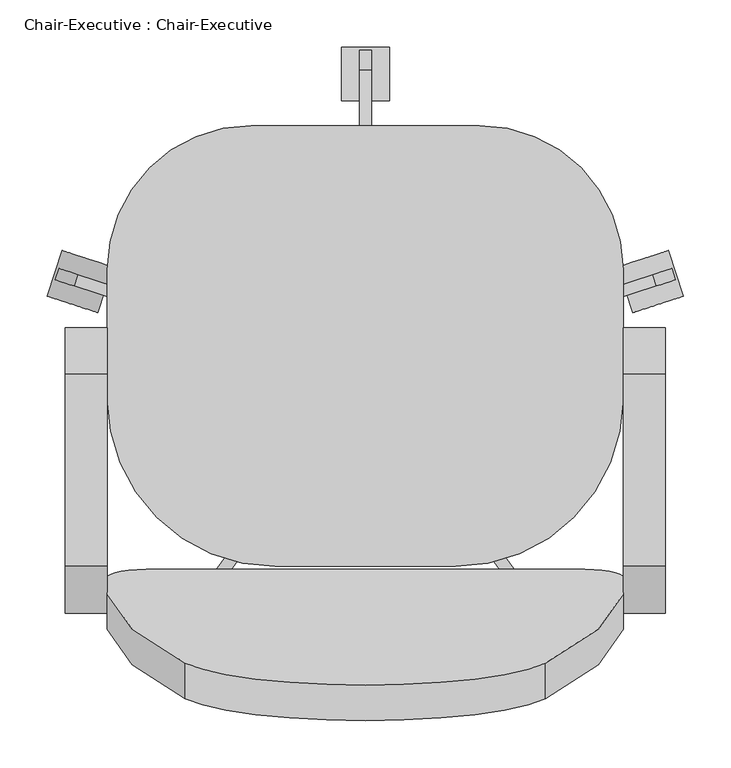
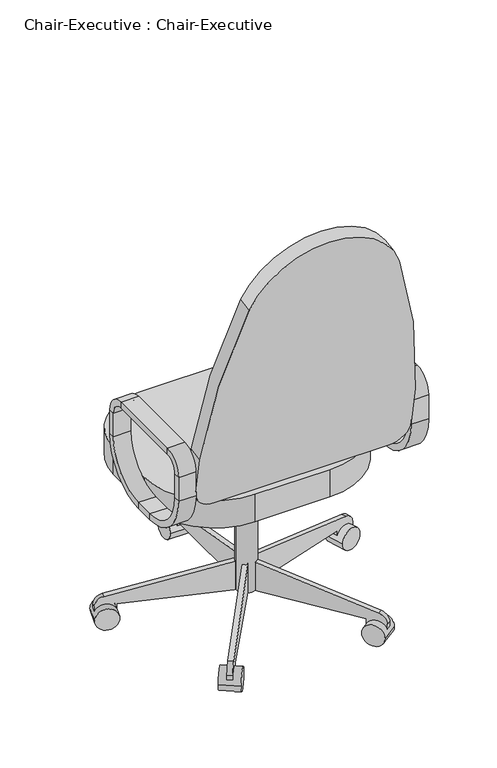
"""IFC4 building model written with IfcOpenShell, lengths in millimetres: furniture geometry, Chair-Executive : Chair-Executive."""

from ifc_helpers import new_model, si_unit, point, frame, frame_2d, origin, place, context, project, spatial, polyline, circle_curve, trimmed, segment, composite_curve, outline, extrude, source, transform, mapped, element, save
from ifc_brep_helpers import plane_surface, cylinder_surface, revolved_surface, advanced_brep


def chair_executive_chair_executive_8d69e98c(model_context):
    return source(origin(), model_context, "Body", "SolidModel", [
        advanced_brep(
        [(-176.5091803, -217.7873012, 546.1), (-176.5091803, -108.0540984, 436.3667972), (-176.5091803, -108.0540984, 420.4917972), (-176.5091803, -233.6623012, 546.1), (-132.0591803, -217.7873012, 546.1), (-132.0591803, -108.0540984, 436.3667972), (-132.0591803, -233.6623012, 546.1), (-132.0591803, -108.0540984, 420.4917972), (-176.5091803, -233.6623012, 609.6), (-176.5091803, -217.7873012, 609.6), (-132.0591803, -217.7873012, 609.6), (-132.0591803, -233.6623012, 609.6), (-176.5091803, -184.2540984, 643.1332028), (-176.5091803, -184.2540984, 659.0082028), (-132.0591803, -184.2540984, 643.1332028), (-132.0591803, -184.2540984, 659.0082028), (-176.5091803, 18.9459016, 659.0082028), (-176.5091803, 18.9459016, 643.1332028), (-132.0591803, 18.9459016, 643.1332028), (-132.0591803, 18.9459016, 659.0082028), (-176.5091803, 52.4791044, 609.6), (-176.5091803, 68.3541044, 609.6), (-132.0591803, 52.4791044, 609.6), (-132.0591803, 68.3541044, 609.6), (-176.5091803, 68.3541044, 546.1), (-176.5091803, 52.4791044, 546.1), (-132.0591803, 52.4791044, 546.1), (-132.0591803, 68.3541044, 546.1), (-176.5091803, -57.2540984, 436.3667972), (-176.5091803, -57.2540984, 420.4917972), (-132.0591803, -57.2540984, 436.3667972), (-132.0591803, -57.2540984, 420.4917972)],
        [
            (0, 1, circle_curve(frame((-176.5091803, -108.0540984, 546.1), z_axis=(1.0, 0.0, 0.0), x_axis=(0.0, 0.0, -1.0)), 109.7332028)),
            (1, 2),
            (2, 3, circle_curve(frame((-176.5091803, -108.0540984, 546.1), z_axis=(-1.0, 0.0, 0.0), x_axis=(0.0, 0.0, -1.0)), 125.6082028)),
            (3, 0),
            (4, 5, circle_curve(frame((-132.0591803, -108.0540984, 546.1), z_axis=(1.0, 0.0, 0.0), x_axis=(0.0, 0.0, -1.0)), 109.7332028)),
            (5, 1),
            (0, 4),
            (6, 7, circle_curve(frame((-132.0591803, -108.0540984, 546.1), z_axis=(1.0, 0.0, 0.0), x_axis=(0.0, 0.0, -1.0)), 125.6082028)),
            (7, 5),
            (4, 6),
            (2, 7),
            (6, 3),
            (3, 8),
            (8, 9),
            (9, 0),
            (9, 10),
            (10, 4),
            (10, 11),
            (11, 6),
            (11, 8),
            (12, 9, circle_curve(frame((-176.5091803, -184.2540984, 609.6), z_axis=(1.0, 0.0, 0.0), x_axis=(0.0, -1.0, 0.0)), 33.5332028)),
            (8, 13, circle_curve(frame((-176.5091803, -184.2540984, 609.6), z_axis=(-1.0, 0.0, 0.0), x_axis=(0.0, -1.0, 0.0)), 49.4082028)),
            (13, 12),
            (14, 10, circle_curve(frame((-132.0591803, -184.2540984, 609.6), z_axis=(1.0, 0.0, 0.0), x_axis=(0.0, -1.0, 0.0)), 33.5332028)),
            (12, 14),
            (15, 11, circle_curve(frame((-132.0591803, -184.2540984, 609.6), z_axis=(1.0, 0.0, 0.0), x_axis=(0.0, -1.0, 0.0)), 49.4082028)),
            (14, 15),
            (15, 13),
            (13, 16),
            (16, 17),
            (17, 12),
            (17, 18),
            (18, 14),
            (18, 19),
            (19, 15),
            (19, 16),
            (20, 17, circle_curve(frame((-176.5091803, 18.9459016, 609.6), z_axis=(1.0, 0.0, 0.0), x_axis=(0.0, 0.0, 1.0)), 33.5332028)),
            (16, 21, circle_curve(frame((-176.5091803, 18.9459016, 609.6), z_axis=(-1.0, 0.0, 0.0), x_axis=(0.0, 0.0, 1.0)), 49.4082028)),
            (21, 20),
            (22, 18, circle_curve(frame((-132.0591803, 18.9459016, 609.6), z_axis=(1.0, 0.0, 0.0), x_axis=(0.0, 0.0, 1.0)), 33.5332028)),
            (20, 22),
            (23, 19, circle_curve(frame((-132.0591803, 18.9459016, 609.6), z_axis=(1.0, 0.0, 0.0), x_axis=(0.0, 0.0, 1.0)), 49.4082028)),
            (22, 23),
            (23, 21),
            (21, 24),
            (24, 25),
            (25, 20),
            (25, 26),
            (26, 22),
            (26, 27),
            (27, 23),
            (27, 24),
            (28, 25, circle_curve(frame((-176.5091803, -57.2540984, 546.1), z_axis=(1.0, 0.0, 0.0), x_axis=(0.0, 1.0, 0.0)), 109.7332028)),
            (24, 29, circle_curve(frame((-176.5091803, -57.2540984, 546.1), z_axis=(-1.0, 0.0, 0.0), x_axis=(0.0, 1.0, 0.0)), 125.6082028)),
            (29, 28),
            (30, 26, circle_curve(frame((-132.0591803, -57.2540984, 546.1), z_axis=(1.0, 0.0, 0.0), x_axis=(0.0, 1.0, 0.0)), 109.7332028)),
            (28, 30),
            (31, 27, circle_curve(frame((-132.0591803, -57.2540984, 546.1), z_axis=(1.0, 0.0, 0.0), x_axis=(0.0, 1.0, 0.0)), 125.6082028)),
            (30, 31),
            (31, 29),
            (29, 2),
            (1, 28),
            (5, 30),
            (7, 31),
        ],
        [
            plane_surface(frame((-176.5091803, -108.0540984, 546.1), z_axis=(-1.0, 0.0, 0.0), x_axis=(0.0, 0.0, -1.0))),
            revolved_surface(polyline([(-176.5091803, -108.0540984, 436.3667972), (-132.0591803, -108.0540984, 436.3667972)]), (-132.0591803, -108.0540984, 546.1), (-1.0, 0.0, 0.0)),
            plane_surface(frame((-132.0591803, -108.0540984, 546.1), z_axis=(1.0, 0.0, 0.0), x_axis=(0.0, 0.0, -1.0))),
            cylinder_surface(frame((-132.0591803, -108.0540984, 546.1), z_axis=(-1.0, 0.0, 0.0), x_axis=(0.0, 0.0, -1.0)), 125.6082028),
            plane_surface(frame((-176.5091803, -233.6623012, 546.1), z_axis=(-1.0, 0.0, 0.0), x_axis=(0.0, 0.0, 1.0))),
            plane_surface(frame((-176.5091803, -217.7873012, 546.1), z_axis=(0.0, 1.0, 0.0), x_axis=(0.0, 0.0, 1.0))),
            plane_surface(frame((-132.0591803, -217.7873012, 546.1), z_axis=(1.0, 0.0, 0.0), x_axis=(0.0, 0.0, 1.0))),
            plane_surface(frame((-132.0591803, -233.6623012, 546.1), z_axis=(0.0, -1.0, 0.0), x_axis=(0.0, 0.0, 1.0))),
            plane_surface(frame((-176.5091803, -184.2540984, 609.6), z_axis=(-1.0, 0.0, 0.0), x_axis=(0.0, -1.0, 0.0))),
            revolved_surface(polyline([(-176.5091803, -217.7873012, 609.6), (-132.0591803, -217.7873012, 609.6)]), (-132.0591803, -184.2540984, 609.6), (-1.0, 0.0, 0.0)),
            plane_surface(frame((-132.0591803, -184.2540984, 609.6), z_axis=(1.0, 0.0, 0.0), x_axis=(0.0, -1.0, 0.0))),
            cylinder_surface(frame((-132.0591803, -184.2540984, 609.6), z_axis=(-1.0, 0.0, 0.0), x_axis=(0.0, -1.0, 0.0)), 49.4082028),
            plane_surface(frame((-176.5091803, -184.2540984, 659.0082028), z_axis=(-1.0, 0.0, 0.0), x_axis=(0.0, 1.0, 0.0))),
            plane_surface(frame((-176.5091803, -184.2540984, 643.1332028), z_axis=(0.0, 0.0, -1.0), x_axis=(0.0, 1.0, 0.0))),
            plane_surface(frame((-132.0591803, -184.2540984, 643.1332028), z_axis=(1.0, 0.0, 0.0), x_axis=(0.0, 1.0, 0.0))),
            plane_surface(frame((-132.0591803, -184.2540984, 659.0082028), z_axis=(0.0, 0.0, 1.0), x_axis=(0.0, 1.0, 0.0))),
            plane_surface(frame((-176.5091803, 18.9459016, 609.6), z_axis=(-1.0, 0.0, 0.0), x_axis=(0.0, 0.0, 1.0))),
            revolved_surface(polyline([(-176.5091803, 18.9459016, 643.1332028), (-132.0591803, 18.9459016, 643.1332028)]), (-132.0591803, 18.9459016, 609.6), (-1.0, 0.0, 0.0)),
            plane_surface(frame((-132.0591803, 18.9459016, 609.6), z_axis=(1.0, 0.0, 0.0), x_axis=(0.0, 0.0, 1.0))),
            cylinder_surface(frame((-132.0591803, 18.9459016, 609.6), z_axis=(-1.0, 0.0, 0.0), x_axis=(0.0, 0.0, 1.0)), 49.4082028),
            plane_surface(frame((-176.5091803, 68.3541044, 609.6), z_axis=(-1.0, 0.0, 0.0), x_axis=(0.0, 0.0, -1.0))),
            plane_surface(frame((-176.5091803, 52.4791044, 609.6), z_axis=(0.0, -1.0, 0.0), x_axis=(0.0, 0.0, -1.0))),
            plane_surface(frame((-132.0591803, 52.4791044, 609.6), z_axis=(1.0, 0.0, 0.0), x_axis=(0.0, 0.0, -1.0))),
            plane_surface(frame((-132.0591803, 68.3541044, 609.6), z_axis=(0.0, 1.0, 0.0), x_axis=(0.0, 0.0, -1.0))),
            plane_surface(frame((-176.5091803, -57.2540984, 546.1), z_axis=(-1.0, 0.0, 0.0), x_axis=(0.0, 1.0, 0.0))),
            revolved_surface(polyline([(-176.5091803, 52.479104400000004, 546.1), (-132.0591803, 52.479104400000004, 546.1)]), (-132.0591803, -57.2540984, 546.1), (-1.0, 0.0, 0.0)),
            plane_surface(frame((-132.0591803, -57.2540984, 546.1), z_axis=(1.0, 0.0, 0.0), x_axis=(0.0, 1.0, 0.0))),
            cylinder_surface(frame((-132.0591803, -57.2540984, 546.1), z_axis=(-1.0, 0.0, 0.0), x_axis=(0.0, 1.0, 0.0)), 125.6082028),
            plane_surface(frame((-176.5091803, -57.2540984, 420.4917972), z_axis=(-1.0, 0.0, 0.0), x_axis=(0.0, -1.0, 0.0))),
            plane_surface(frame((-176.5091803, -57.2540984, 436.3667972), z_axis=(0.0, 0.0, 1.0), x_axis=(0.0, -1.0, 0.0))),
            plane_surface(frame((-132.0591803, -57.2540984, 436.3667972), z_axis=(1.0, 0.0, 0.0), x_axis=(0.0, -1.0, 0.0))),
            plane_surface(frame((-132.0591803, -57.2540984, 420.4917972), z_axis=(0.0, 0.0, -1.0), x_axis=(0.0, -1.0, 0.0))),
        ],
        [
            (0, [[1, 2, 3, 4]]),
            (1, [[5, 6, -1, 7]]),
            (2, [[8, 9, -5, 10]]),
            (3, [[-3, 11, -8, 12]]),
            (4, [[-4, 13, 14, 15]]),
            (5, [[-7, -15, 16, 17]]),
            (6, [[-10, -17, 18, 19]]),
            (7, [[-12, -19, 20, -13]]),
            (8, [[21, -14, 22, 23]]),
            (9, [[24, -16, -21, 25]]),
            (10, [[26, -18, -24, 27]]),
            (11, [[-22, -20, -26, 28]]),
            (12, [[-23, 29, 30, 31]]),
            (13, [[-25, -31, 32, 33]]),
            (14, [[-27, -33, 34, 35]]),
            (15, [[-28, -35, 36, -29]]),
            (16, [[37, -30, 38, 39]]),
            (17, [[40, -32, -37, 41]]),
            (18, [[42, -34, -40, 43]]),
            (19, [[-38, -36, -42, 44]]),
            (20, [[-39, 45, 46, 47]]),
            (21, [[-41, -47, 48, 49]]),
            (22, [[-43, -49, 50, 51]]),
            (23, [[-44, -51, 52, -45]]),
            (24, [[53, -46, 54, 55]]),
            (25, [[56, -48, -53, 57]]),
            (26, [[58, -50, -56, 59]]),
            (27, [[-54, -52, -58, 60]]),
            (28, [[-55, 61, -2, 62]]),
            (29, [[-57, -62, -6, 63]]),
            (30, [[-59, -63, -9, 64]]),
            (31, [[-60, -64, -11, -61]]),
        ],
    ),
        advanced_brep(
        [(414.0408197, -233.6623012, 546.1), (414.0408197, -108.0540984, 420.4917972), (458.4908197, -108.0540984, 420.4917972), (458.4908197, -233.6623012, 546.1), (414.0408197, -217.7873012, 546.1), (414.0408197, -108.0540984, 436.3667972), (458.4908197, -217.7873012, 546.1), (458.4908197, -108.0540984, 436.3667972), (458.4908197, -233.6623012, 609.6), (414.0408197, -233.6623012, 609.6), (414.0408197, -217.7873012, 609.6), (458.4908197, -217.7873012, 609.6), (414.0408197, -184.2540984, 659.0082028), (458.4908197, -184.2540984, 659.0082028), (414.0408197, -184.2540984, 643.1332028), (458.4908197, -184.2540984, 643.1332028), (458.4908197, 18.9459016, 659.0082028), (414.0408197, 18.9459016, 659.0082028), (414.0408197, 18.9459016, 643.1332028), (458.4908197, 18.9459016, 643.1332028), (414.0408197, 68.3541044, 609.6), (458.4908197, 68.3541044, 609.6), (414.0408197, 52.4791044, 609.6), (458.4908197, 52.4791044, 609.6), (458.4908197, 68.3541044, 546.1), (414.0408197, 68.3541044, 546.1), (414.0408197, 52.4791044, 546.1), (458.4908197, 52.4791044, 546.1), (414.0408197, -57.2540984, 420.4917972), (458.4908197, -57.2540984, 420.4917972), (414.0408197, -57.2540984, 436.3667972), (458.4908197, -57.2540984, 436.3667972)],
        [
            (0, 1, circle_curve(frame((414.0408197, -108.0540984, 546.1), z_axis=(1.0, 0.0, 0.0), x_axis=(0.0, 0.0, -1.0)), 125.6082028)),
            (1, 2),
            (2, 3, circle_curve(frame((458.4908197, -108.0540984, 546.1), z_axis=(-1.0, 0.0, 0.0), x_axis=(0.0, 0.0, -1.0)), 125.6082028)),
            (3, 0),
            (4, 5, circle_curve(frame((414.0408197, -108.0540984, 546.1), z_axis=(1.0, 0.0, 0.0), x_axis=(0.0, 0.0, -1.0)), 109.7332028)),
            (5, 1),
            (0, 4),
            (6, 7, circle_curve(frame((458.4908197, -108.0540984, 546.1), z_axis=(1.0, 0.0, 0.0), x_axis=(0.0, 0.0, -1.0)), 109.7332028)),
            (7, 5),
            (4, 6),
            (2, 7),
            (6, 3),
            (3, 8),
            (8, 9),
            (9, 0),
            (9, 10),
            (10, 4),
            (10, 11),
            (11, 6),
            (11, 8),
            (12, 9, circle_curve(frame((414.0408197, -184.2540984, 609.6), z_axis=(1.0, 0.0, 0.0), x_axis=(0.0, -1.0, 0.0)), 49.4082028)),
            (8, 13, circle_curve(frame((458.4908197, -184.2540984, 609.6), z_axis=(-1.0, 0.0, 0.0), x_axis=(0.0, -1.0, 0.0)), 49.4082028)),
            (13, 12),
            (14, 10, circle_curve(frame((414.0408197, -184.2540984, 609.6), z_axis=(1.0, 0.0, 0.0), x_axis=(0.0, -1.0, 0.0)), 33.5332028)),
            (12, 14),
            (15, 11, circle_curve(frame((458.4908197, -184.2540984, 609.6), z_axis=(1.0, 0.0, 0.0), x_axis=(0.0, -1.0, 0.0)), 33.5332028)),
            (14, 15),
            (15, 13),
            (13, 16),
            (16, 17),
            (17, 12),
            (17, 18),
            (18, 14),
            (18, 19),
            (19, 15),
            (19, 16),
            (20, 17, circle_curve(frame((414.0408197, 18.9459016, 609.6), z_axis=(1.0, 0.0, 0.0), x_axis=(0.0, 0.0, 1.0)), 49.4082028)),
            (16, 21, circle_curve(frame((458.4908197, 18.9459016, 609.6), z_axis=(-1.0, 0.0, 0.0), x_axis=(0.0, 0.0, 1.0)), 49.4082028)),
            (21, 20),
            (22, 18, circle_curve(frame((414.0408197, 18.9459016, 609.6), z_axis=(1.0, 0.0, 0.0), x_axis=(0.0, 0.0, 1.0)), 33.5332028)),
            (20, 22),
            (23, 19, circle_curve(frame((458.4908197, 18.9459016, 609.6), z_axis=(1.0, 0.0, 0.0), x_axis=(0.0, 0.0, 1.0)), 33.5332028)),
            (22, 23),
            (23, 21),
            (21, 24),
            (24, 25),
            (25, 20),
            (25, 26),
            (26, 22),
            (26, 27),
            (27, 23),
            (27, 24),
            (28, 25, circle_curve(frame((414.0408197, -57.2540984, 546.1), z_axis=(1.0, 0.0, 0.0), x_axis=(0.0, 1.0, 0.0)), 125.6082028)),
            (24, 29, circle_curve(frame((458.4908197, -57.2540984, 546.1), z_axis=(-1.0, 0.0, 0.0), x_axis=(0.0, 1.0, 0.0)), 125.6082028)),
            (29, 28),
            (30, 26, circle_curve(frame((414.0408197, -57.2540984, 546.1), z_axis=(1.0, 0.0, 0.0), x_axis=(0.0, 1.0, 0.0)), 109.7332028)),
            (28, 30),
            (31, 27, circle_curve(frame((458.4908197, -57.2540984, 546.1), z_axis=(1.0, 0.0, 0.0), x_axis=(0.0, 1.0, 0.0)), 109.7332028)),
            (30, 31),
            (31, 29),
            (29, 2),
            (1, 28),
            (5, 30),
            (7, 31),
        ],
        [
            cylinder_surface(frame((414.0408197, -108.0540984, 546.1), z_axis=(-1.0, 0.0, 0.0), x_axis=(0.0, 0.0, -1.0)), 125.6082028),
            plane_surface(frame((414.0408197, -108.0540984, 546.1), z_axis=(-1.0, 0.0, 0.0), x_axis=(0.0, 0.0, -1.0))),
            revolved_surface(polyline([(414.0408197, -108.0540984, 436.3667972), (458.4908197, -108.0540984, 436.3667972)]), (414.0408197, -108.0540984, 546.1), (-1.0, 0.0, 0.0)),
            plane_surface(frame((458.4908197, -108.0540984, 546.1), z_axis=(1.0, 0.0, 0.0), x_axis=(0.0, 0.0, -1.0))),
            plane_surface(frame((458.4908197, -233.6623012, 546.1), z_axis=(0.0, -1.0, 0.0), x_axis=(0.0, 0.0, 1.0))),
            plane_surface(frame((414.0408197, -233.6623012, 546.1), z_axis=(-1.0, 0.0, 0.0), x_axis=(0.0, 0.0, 1.0))),
            plane_surface(frame((414.0408197, -217.7873012, 546.1), z_axis=(0.0, 1.0, 0.0), x_axis=(0.0, 0.0, 1.0))),
            plane_surface(frame((458.4908197, -217.7873012, 546.1), z_axis=(1.0, 0.0, 0.0), x_axis=(0.0, 0.0, 1.0))),
            cylinder_surface(frame((414.0408197, -184.2540984, 609.6), z_axis=(-1.0, 0.0, 0.0), x_axis=(0.0, -1.0, 0.0)), 49.4082028),
            plane_surface(frame((414.0408197, -184.2540984, 609.6), z_axis=(-1.0, 0.0, 0.0), x_axis=(0.0, -1.0, 0.0))),
            revolved_surface(polyline([(414.0408197, -217.7873012, 609.6), (458.4908197, -217.7873012, 609.6)]), (414.0408197, -184.2540984, 609.6), (-1.0, 0.0, 0.0)),
            plane_surface(frame((458.4908197, -184.2540984, 609.6), z_axis=(1.0, 0.0, 0.0), x_axis=(0.0, -1.0, 0.0))),
            plane_surface(frame((458.4908197, -184.2540984, 659.0082028), z_axis=(0.0, 0.0, 1.0), x_axis=(0.0, 1.0, 0.0))),
            plane_surface(frame((414.0408197, -184.2540984, 659.0082028), z_axis=(-1.0, 0.0, 0.0), x_axis=(0.0, 1.0, 0.0))),
            plane_surface(frame((414.0408197, -184.2540984, 643.1332028), z_axis=(0.0, 0.0, -1.0), x_axis=(0.0, 1.0, 0.0))),
            plane_surface(frame((458.4908197, -184.2540984, 643.1332028), z_axis=(1.0, 0.0, 0.0), x_axis=(0.0, 1.0, 0.0))),
            cylinder_surface(frame((414.0408197, 18.9459016, 609.6), z_axis=(-1.0, 0.0, 0.0), x_axis=(0.0, 0.0, 1.0)), 49.4082028),
            plane_surface(frame((414.0408197, 18.9459016, 609.6), z_axis=(-1.0, 0.0, 0.0), x_axis=(0.0, 0.0, 1.0))),
            revolved_surface(polyline([(414.0408197, 18.9459016, 643.1332028), (458.4908197, 18.9459016, 643.1332028)]), (414.0408197, 18.9459016, 609.6), (-1.0, 0.0, 0.0)),
            plane_surface(frame((458.4908197, 18.9459016, 609.6), z_axis=(1.0, 0.0, 0.0), x_axis=(0.0, 0.0, 1.0))),
            plane_surface(frame((458.4908197, 68.3541044, 609.6), z_axis=(0.0, 1.0, 0.0), x_axis=(0.0, 0.0, -1.0))),
            plane_surface(frame((414.0408197, 68.3541044, 609.6), z_axis=(-1.0, 0.0, 0.0), x_axis=(0.0, 0.0, -1.0))),
            plane_surface(frame((414.0408197, 52.4791044, 609.6), z_axis=(0.0, -1.0, 0.0), x_axis=(0.0, 0.0, -1.0))),
            plane_surface(frame((458.4908197, 52.4791044, 609.6), z_axis=(1.0, 0.0, 0.0), x_axis=(0.0, 0.0, -1.0))),
            cylinder_surface(frame((414.0408197, -57.2540984, 546.1), z_axis=(-1.0, 0.0, 0.0), x_axis=(0.0, 1.0, 0.0)), 125.6082028),
            plane_surface(frame((414.0408197, -57.2540984, 546.1), z_axis=(-1.0, 0.0, 0.0), x_axis=(0.0, 1.0, 0.0))),
            revolved_surface(polyline([(414.0408197, 52.479104400000004, 546.1), (458.4908197, 52.479104400000004, 546.1)]), (414.0408197, -57.2540984, 546.1), (-1.0, 0.0, 0.0)),
            plane_surface(frame((458.4908197, -57.2540984, 546.1), z_axis=(1.0, 0.0, 0.0), x_axis=(0.0, 1.0, 0.0))),
            plane_surface(frame((458.4908197, -57.2540984, 420.4917972), z_axis=(0.0, 0.0, -1.0), x_axis=(0.0, -1.0, 0.0))),
            plane_surface(frame((414.0408197, -57.2540984, 420.4917972), z_axis=(-1.0, 0.0, 0.0), x_axis=(0.0, -1.0, 0.0))),
            plane_surface(frame((414.0408197, -57.2540984, 436.3667972), z_axis=(0.0, 0.0, 1.0), x_axis=(0.0, -1.0, 0.0))),
            plane_surface(frame((458.4908197, -57.2540984, 436.3667972), z_axis=(1.0, 0.0, 0.0), x_axis=(0.0, -1.0, 0.0))),
        ],
        [
            (0, [[1, 2, 3, 4]]),
            (1, [[5, 6, -1, 7]]),
            (2, [[8, 9, -5, 10]]),
            (3, [[-3, 11, -8, 12]]),
            (4, [[-4, 13, 14, 15]]),
            (5, [[-7, -15, 16, 17]]),
            (6, [[-10, -17, 18, 19]]),
            (7, [[-12, -19, 20, -13]]),
            (8, [[21, -14, 22, 23]]),
            (9, [[24, -16, -21, 25]]),
            (10, [[26, -18, -24, 27]]),
            (11, [[-22, -20, -26, 28]]),
            (12, [[-23, 29, 30, 31]]),
            (13, [[-25, -31, 32, 33]]),
            (14, [[-27, -33, 34, 35]]),
            (15, [[-28, -35, 36, -29]]),
            (16, [[37, -30, 38, 39]]),
            (17, [[40, -32, -37, 41]]),
            (18, [[42, -34, -40, 43]]),
            (19, [[-38, -36, -42, 44]]),
            (20, [[-39, 45, 46, 47]]),
            (21, [[-41, -47, 48, 49]]),
            (22, [[-43, -49, 50, 51]]),
            (23, [[-44, -51, 52, -45]]),
            (24, [[53, -46, 54, 55]]),
            (25, [[56, -48, -53, 57]]),
            (26, [[58, -50, -56, 59]]),
            (27, [[-54, -52, -58, 60]]),
            (28, [[-55, 61, -2, 62]]),
            (29, [[-57, -62, -6, 63]]),
            (30, [[-59, -63, -9, 64]]),
            (31, [[-60, -64, -11, -61]]),
        ],
    ),
        extrude(outline(composite_curve([segment(trimmed(circle_curve(frame_2d((0.0, -50.8)), 50.8), [point((0.0, 0.0))], [point((50.8, -50.8))], False, "CARTESIAN"), True, "CONTINUOUS"), segment(polyline([(50.8, -50.8), (50.8, -152.4)]), True, "CONTINUOUS"), segment(trimmed(circle_curve(frame_2d((-1471.2021854, -74.3913617)), 1524.0), [point((50.8, -152.4))], [point((-31.75, -574.9444618))], False, "CARTESIAN"), True, "CONTINUOUS"), segment(trimmed(circle_curve(frame_2d((-222.25, -504.2338544)), 203.2), [point((-31.75, -574.9444618))], [point((-412.75, -574.9444618))], False, "CARTESIAN"), True, "CONTINUOUS"), segment(trimmed(circle_curve(frame_2d((1026.7021854, -74.3913617)), 1524.0), [point((-412.75, -574.9444618))], [point((-495.3, -152.4))], False, "CARTESIAN"), True, "CONTINUOUS"), segment(polyline([(-495.3, -152.4), (-495.3, -50.8)]), True, "CONTINUOUS"), segment(trimmed(circle_curve(frame_2d((-444.5, -50.8)), 50.8), [point((-495.3, -50.8))], [point((-444.5, 0.0))], False, "CARTESIAN"), True, "CONTINUOUS"), segment(polyline([(-444.5, 0.0), (0.0, 0.0)]), True, "CONTINUOUS")], self_intersect=False)), frame((363.2408197, -224.5698964, 503.1641822), z_axis=(0.0, 0.9848077530122084, 0.17364817766692853), x_axis=(1.0, 0.0, 0.0)), (0.0, 0.0, 1.0), 38.1),
        extrude(outline(composite_curve([segment(trimmed(circle_curve(frame_2d((20.3408197, 129.4961016)), 152.4), [point((-132.0591803, 129.4961016))], [point((20.3408197, 281.8961016))], False, "CARTESIAN"), True, "CONTINUOUS"), segment(polyline([(20.3408197, 281.8961016), (261.6408197, 281.8961016)]), True, "CONTINUOUS"), segment(trimmed(circle_curve(frame_2d((261.6408197, 129.4961016)), 152.4), [point((261.6408197, 281.8961016))], [point((414.0408197, 129.4961016))], False, "CARTESIAN"), True, "CONTINUOUS"), segment(polyline([(414.0408197, 129.4961016), (414.0408197, -6.4540984)]), True, "CONTINUOUS"), segment(trimmed(circle_curve(frame_2d((236.2408197, -6.4540984)), 177.8), [point((414.0408197, -6.4540984))], [point((236.2408197, -184.2540984))], False, "CARTESIAN"), True, "CONTINUOUS"), segment(polyline([(236.2408197, -184.2540984), (45.7408197, -184.2540984)]), True, "CONTINUOUS"), segment(trimmed(circle_curve(frame_2d((45.7408197, -6.4540984)), 177.8), [point((45.7408197, -184.2540984))], [point((-132.0591803, -6.4540984))], False, "CARTESIAN"), True, "CONTINUOUS"), segment(polyline([(-132.0591803, -6.4540984), (-132.0591803, 129.4961016)]), True, "CONTINUOUS")], self_intersect=False)), frame((0.0, 0.0, 383.7835944), z_axis=(0.0, 0.0, 1.0), x_axis=(1.0, 0.0, 0.0)), (0.0, 0.0, 1.0), 73.4164056),
        extrude(outline(composite_curve([segment(trimmed(circle_curve(frame_2d((140.9908197, 18.9459016)), 25.4), [point((115.5908197, 18.9459016))], [point((166.3908197, 18.9459016))], False, "CARTESIAN"), True, "CONTINUOUS"), segment(trimmed(circle_curve(frame_2d((140.9908197, 18.9459016)), 25.4), [point((166.3908197, 18.9459016))], [point((115.5908197, 18.9459016))], False, "CARTESIAN"), True, "CONTINUOUS")], self_intersect=False)), frame((0.0, 0.0, 53.5835944), z_axis=(0.0, 0.0, 1.0), x_axis=(1.0, 0.0, 0.0)), (0.0, 0.0, 1.0), 330.5914056),
        extrude(outline(composite_curve([segment(trimmed(circle_curve(frame_2d((0.0, -28.2002727)), 28.2002727), [point((0.0, -56.4005455))], [point((0.0, 0.0))], False, "CARTESIAN"), True, "CONTINUOUS"), segment(trimmed(circle_curve(frame_2d((0.0, -28.2002727)), 28.2002727), [point((0.0, 0.0))], [point((0.0, -56.4005455))], False, "CARTESIAN"), True, "CONTINUOUS")], self_intersect=False)), frame((477.6203484, 101.6163254, 28.1835944), z_axis=(-0.3090169943749423, 0.9510565162951553, 0.0), x_axis=(0.0, 0.0, 1.0)), (0.0, 0.0, 1.0), 50.8),
        extrude(outline(composite_curve([segment(polyline([(-25.4, 0.0), (0.0, 0.0), (0.0, -50.8), (-24.303053, -50.8)]), True, "CONTINUOUS"), segment(trimmed(circle_curve(frame_2d((-24.303053, -25.4)), 25.4), [point((-24.303053, -50.8))], [point((-49.3171699, -29.8106637))], False, "CARTESIAN"), True, "CONTINUOUS"), segment(polyline([(-49.3171699, -29.8106637), (-101.6, 266.7), (-101.6, 292.1), (-25.4, 292.1), (-25.4, 0.0)]), True, "CONTINUOUS")], self_intersect=False)), frame((420.756686, 103.1705568, 28.1835944), z_axis=(-0.3090169943749423, 0.9510565162951553, 0.0), x_axis=(0.0, 0.0, -1.0)), (0.0, 0.0, 1.0), 12.7),
        extrude(outline(composite_curve([segment(trimmed(circle_curve(frame_2d((0.0, -28.2002727)), 28.2002727), [point((0.0, -56.4005455))], [point((0.0, 0.0))], False, "CARTESIAN"), True, "CONTINUOUS"), segment(trimmed(circle_curve(frame_2d((0.0, -28.2002727)), 28.2002727), [point((0.0, 0.0))], [point((0.0, -56.4005455))], False, "CARTESIAN"), True, "CONTINUOUS")], self_intersect=False)), frame((323.63931, -275.6612394, 28.1835944), z_axis=(0.8090169943749499, 0.5877852522924699, 0.0), x_axis=(0.0, 0.0, 1.0)), (0.0, 0.0, 1.0), 50.8),
        extrude(outline(composite_curve([segment(polyline([(-25.4, 0.0), (0.0, 0.0), (0.0, -50.8), (-24.303053, -50.8)]), True, "CONTINUOUS"), segment(trimmed(circle_curve(frame_2d((-24.303053, -25.3999999)), 25.4), [point((-24.303053, -50.8))], [point((-49.3171699, -29.8106636))], False, "CARTESIAN"), True, "CONTINUOUS"), segment(polyline([(-49.3171699, -29.8106636), (-101.6, 266.7), (-101.6, 292.1), (-25.4, 292.1), (-25.4, 0.0)]), True, "CONTINUOUS")], self_intersect=False)), frame((307.545634, -221.1003988, 28.1835944), z_axis=(0.8090169943749499, 0.5877852522924699, 0.0), x_axis=(0.0, 0.0, -1.0)), (0.0, 0.0, 1.0), 12.7),
        extrude(outline(composite_curve([segment(trimmed(circle_curve(frame_2d((0.0, -28.2002727)), 28.2002727), [point((0.0, -56.4005455))], [point((0.0, 0.0))], False, "CARTESIAN"), True, "CONTINUOUS"), segment(trimmed(circle_curve(frame_2d((0.0, -28.2002727)), 28.2002727), [point((0.0, 0.0))], [point((0.0, -56.4005455))], False, "CARTESIAN"), True, "CONTINUOUS")], self_intersect=False)), frame((-41.6576707, -275.6612394, 28.1835944), z_axis=(-0.8090169943749458, 0.5877852522924754, 0.0), x_axis=(0.0, 0.0, -1.0)), (0.0, 0.0, 1.0), 50.8),
        extrude(outline(composite_curve([segment(polyline([(25.4, 0.0), (25.4, 292.1), (101.6, 292.1), (101.6, 266.7), (49.3171699, -29.8106637)]), True, "CONTINUOUS"), segment(trimmed(circle_curve(frame_2d((24.303053, -25.3999999)), 25.4), [point((49.3171699, -29.8106637))], [point((24.303053, -50.8))], False, "CARTESIAN"), True, "CONTINUOUS"), segment(polyline([(24.303053, -50.8), (0.0, -50.8), (0.0, 0.0), (25.4, 0.0)]), True, "CONTINUOUS")], self_intersect=False)), frame((-25.5639946, -221.1003988, 28.1835944), z_axis=(-0.8090169943749459, 0.5877852522924754, 0.0), x_axis=(0.0, 0.0, 1.0)), (0.0, 0.0, 1.0), 12.7),
        extrude(outline(composite_curve([segment(trimmed(circle_curve(frame_2d((0.0, -28.2002727)), 28.2002727), [point((0.0, -56.4005454))], [point((0.0, 0.0))], False, "CARTESIAN"), True, "CONTINUOUS"), segment(trimmed(circle_curve(frame_2d((0.0, -28.2002727)), 28.2002727), [point((0.0, 0.0))], [point((0.0, -56.4005454))], False, "CARTESIAN"), True, "CONTINUOUS")], self_intersect=False)), frame((-195.638709, 101.6163254, 28.1835944), z_axis=(0.3090169943749487, 0.9510565162951532, 0.0), x_axis=(0.0, 0.0, -1.0)), (0.0, 0.0, 1.0), 50.8),
        extrude(outline(composite_curve([segment(polyline([(25.4, 0.0), (25.4, 292.1000001), (101.6, 292.1000001), (101.6, 266.7), (49.3171699, -29.8106636)]), True, "CONTINUOUS"), segment(trimmed(circle_curve(frame_2d((24.303053, -25.4)), 25.4), [point((49.3171699, -29.8106636))], [point((24.303053, -50.8))], False, "CARTESIAN"), True, "CONTINUOUS"), segment(polyline([(24.303053, -50.8), (0.0, -50.8), (0.0, 0.0), (25.4, 0.0)]), True, "CONTINUOUS")], self_intersect=False)), frame((-138.7750467, 103.1705568, 28.1835944), z_axis=(0.3090169943749487, 0.9510565162951532, 0.0), x_axis=(0.0, 0.0, 1.0)), (0.0, 0.0, 1.0), 12.7),
        extrude(outline(composite_curve([segment(trimmed(circle_curve(frame_2d((336.4459016, 28.1835944)), 28.2002727), [point((308.2456289, 28.1835944))], [point((364.6461744, 28.1835944))], False, "CARTESIAN"), True, "CONTINUOUS"), segment(trimmed(circle_curve(frame_2d((336.4459016, 28.1835944)), 28.2002727), [point((364.6461744, 28.1835944))], [point((308.2456289, 28.1835944))], False, "CARTESIAN"), True, "CONTINUOUS")], self_intersect=False)), frame((115.5908197, 0.0, 0.0), z_axis=(1.0, 0.0, 0.0), x_axis=(0.0, 1.0, 0.0)), (0.0, 0.0, 1.0), 50.8),
        extrude(outline(composite_curve([segment(polyline([(311.0459016, 53.5835944), (18.9459016, 53.5835944), (18.9459016, 129.7835944), (44.3459016, 129.7835944), (340.8565654, 77.5007643)]), True, "CONTINUOUS"), segment(trimmed(circle_curve(frame_2d((336.4459016, 52.4866474)), 25.4), [point((340.8565654, 77.5007643))], [point((361.8459016, 52.4866474))], False, "CARTESIAN"), True, "CONTINUOUS"), segment(polyline([(361.8459016, 52.4866474), (361.8459016, 28.1835944), (311.0459016, 28.1835944), (311.0459016, 53.5835944)]), True, "CONTINUOUS")], self_intersect=False)), frame((134.6408197, 0.0, 0.0), z_axis=(1.0, 0.0, 0.0), x_axis=(0.0, 1.0, 0.0)), (0.0, 0.0, 1.0), 12.7),
        extrude(outline(polyline([(69.7459016, 383.7835944), (69.7459016, 371.0835944), (18.9459016, 283.0954134), (-19.1540984, 283.0954134), (-19.1540984, 383.7835944), (69.7459016, 383.7835944)])), frame((90.1908197, 0.0, 0.0), z_axis=(1.0, 0.0, 0.0), x_axis=(0.0, 1.0, 0.0)), (0.0, 0.0, 1.0), 101.6),
    ])


if __name__ == "__main__":
    model = new_model("IFC4")
    model_context = context("Model", 3, world=origin())
    ifc_project = project(units=[si_unit("LENGTHUNIT", "METRE", prefix="MILLI")], contexts=[model_context])
    site = spatial("IfcSite", under=ifc_project)
    building = spatial("IfcBuilding", under=site)
    placement = place(None, origin())
    chair_executive_chair_executive_shape = chair_executive_chair_executive_8d69e98c(model_context)
    element("IfcFurniture", 1, ObjectType="Chair-Executive : Chair-Executive", at=placement, inside=building, context=model_context, shape_type="MappedRepresentation", body=[
        mapped(chair_executive_chair_executive_shape, transform((0.0, 0.0, 0.0), x_axis=(1.0, 0.0, 0.0), y_axis=(0.0, 1.0, 0.0), z_axis=(0.0, 0.0, 1.0))),
    ])
    save(model, "model.ifc")

# Revit data of these elements
# Type "Chair-Executive : Chair-Executive"
#   Assembly Code = "E2020200"
#   Base/Arms Material = Plastic, Opaque Black
#   Casters Material = Plastic, Opaque Black
#   Seat/Back Material = Textile - Slate Blue
#   Default Elevation = 0
# Element 1 (IfcFurniture, "Chair-Executive : Chair-Executive")
#   Materials on its faces: "Plastic, Opaque Black", "Textile - Slate Blue"
# Materials
#   "Plastic, Opaque Black": class "Plastic", colour RGB 0 0 0, transparency 0, Description = "Plastic, generic, opaque black", Cost = 0
#   "Textile - Slate Blue": class "Fabric", colour RGB 98 102 118, transparency 0
